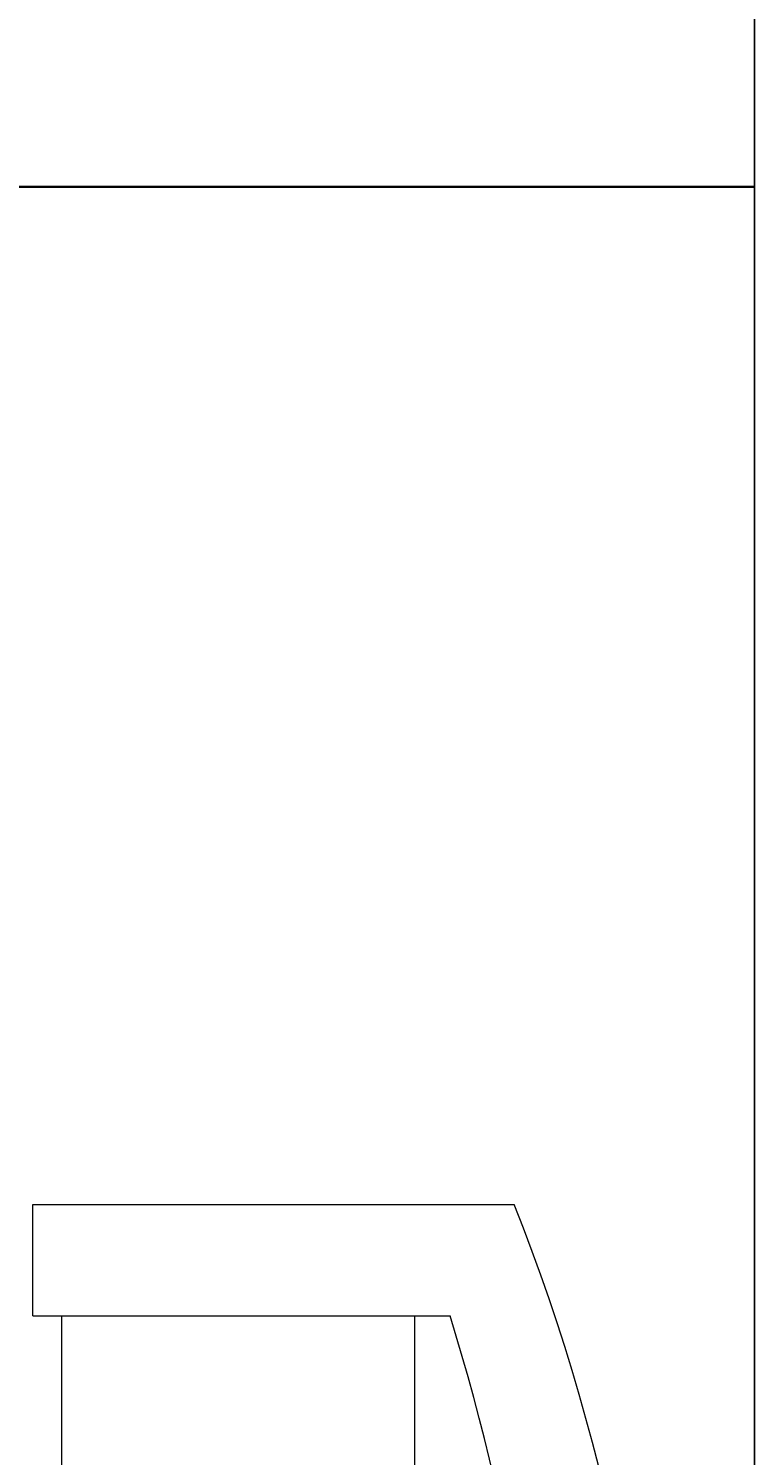
# Model space of a CAD drawing. Units: feet. Extents: x 1654 to 2985, y 1348 to 2230.
# Tile 51 of 53: x 2759 to 2785, y 1842 to 1892. Entities that reach past the tile are written whole.
import ezdxf

# ---------------------------------------------------------------- set-up
doc = ezdxf.new("R2010")
doc.units = ezdxf.units.FT
for name, color, linetype, lineweight in [('A-ANNO-DIMS', 2, 'Continuous', 18), ('A-FURN', 8, 'Continuous', 13), ('A-WALL', 7, 'Continuous', 35)]:
    doc.layers.add(name, color=color, linetype=linetype, lineweight=lineweight)
doc.styles.get("Standard").update_dxf_attribs({"font": 'arial.ttf'})
doc.dimstyles.get("Standard").update_dxf_attribs({"dimtxt": 0.18, "dimasz": 0.18, "dimexe": 0.18, "dimexo": 0.0625, "dimgap": 0.09, "dimtad": 0, "dimtih": 1, "dimtoh": 1, "dimdec": 4, "dimzin": 0, "dimdsep": 46, "dimtxsty": 'Standard', "dimcen": 0.09, "dimadec": 0, "dimazin": 0, "dimtfac": 1, "dimtdec": 4, "dimtofl": 0, "dimtmove": 0, "dimatfit": 3, "dimfxl": 1, "dimtolj": 1, "dimtzin": 0, "dimarcsym": 0})

# ---------------------------------------------------------------- blocks, each defined once
blk = doc.blocks.new('Sofa - Roundback 7 ft.')
for p, q in [((-36.000027, -34), (-36.000027, -11.4696)), ((-35.999844, -13.3819), (35.9998, -13.3819)), ((-36.000027, -32.4421), (35.99998, -32.4421))]:
    blk.add_line(p, q)
blk.add_lwpolyline([(-36.000027, -34), (-42.000027, -34), (-42.000027, -8)])
for centre, radius, start, end in [((0, -114.25), 114.25, 68.43141, 111.5686), ((-0.00001, -127.1968), 121.1968, 72.72033, 107.2797)]:
    blk.add_arc(centre, radius, start, end)
blk = doc.blocks.new('*D82')
at = {"layer": 'A-ANNO-DIMS', "color": 0, "lineweight": -2, "transparency": 16777216}
for p, q in [((2652.706, 2039.192), (2652.706, 1490.625)), ((2784.706, 2039.192), (2784.706, 1490.625)), ((2652.886, 1490.805), (2718.426, 1490.805)), ((2784.526, 1490.805), (2718.985, 1490.805))]:
    blk.add_line(p, q, dxfattribs=at)
at = {"layer": 'A-ANNO-DIMS', "color": 0, "transparency": 16777216}
for points in [[(2652.886, 1490.835), (2652.886, 1490.775), (2652.706, 1490.805)], [(2784.526, 1490.835), (2784.526, 1490.775), (2784.706, 1490.805)]]:
    blk.add_solid(points, dxfattribs=at)
at = {"layer": 'Defpoints', "color": 0, "transparency": 16777216}
for p in [(2652.706, 2039.255), (2784.706, 2039.255), (2784.706, 1490.805)]:
    blk.add_point(p, dxfattribs=at)
at = {"layer": 'A-ANNO-DIMS', "color": 0, "transparency": 16777216, "insert": (2718.706, 1490.805), "char_height": 0.18, "attachment_point": 5}
blk.add_mtext('\\A1;132', dxfattribs=at)
blk = doc.blocks.new('*D86')
at = {"layer": 'A-ANNO-DIMS', "color": 0, "lineweight": -2, "transparency": 16777216}
for p, q in [((2748.706, 1616.317), (2748.706, 2149.885)), ((2784.706, 1607.317), (2784.706, 2149.885)), ((2748.886, 2149.705), (2766.487, 2149.705)), ((2784.526, 2149.705), (2766.925, 2149.705))]:
    blk.add_line(p, q, dxfattribs=at)
at = {"layer": 'A-ANNO-DIMS', "color": 0, "transparency": 16777216}
for points in [[(2748.886, 2149.735), (2748.886, 2149.675), (2748.706, 2149.705)], [(2784.526, 2149.735), (2784.526, 2149.675), (2784.706, 2149.705)]]:
    blk.add_solid(points, dxfattribs=at)
at = {"layer": 'Defpoints', "color": 0, "transparency": 16777216}
for p in [(2784.706, 2149.705), (2748.706, 1616.255), (2784.706, 1607.255)]:
    blk.add_point(p, dxfattribs=at)
at = {"layer": 'A-ANNO-DIMS', "color": 0, "transparency": 16777216, "insert": (2766.706, 2149.705), "char_height": 0.18, "attachment_point": 5}
blk.add_mtext('\\A1;36', dxfattribs=at)

msp = doc.modelspace()

# ---------------------------------------------------------------- linework, layer by layer
at = {"layer": 'A-WALL'}
msp.add_line((2784.7058, 1886.2549), (2652.7058, 1886.2549), dxfattribs=at)

# ---------------------------------------------------------------- block references
at = {"layer": 'A-FURN', "xscale": 0.6464854603293951, "yscale": 0.6464854603293951, "zscale": 0.6464854603293951, "rotation": 270}
msp.add_blockref('Sofa - Roundback 7 ft.', (2781.495, 1823.581), dxfattribs=at)

# ---------------------------------------------------------------- dimensions: what is measured, and where the dimension line sits
at = {"layer": 'A-ANNO-DIMS'}
for base, p1, p2, picture, middle in [((2784.7058, 2149.7049), (2748.7058, 1616.2549), (2784.7058, 1607.2549), '*D86', (2766.7058, 2149.7049)), ((2784.7058, 1490.8049), (2652.7058, 2039.2549), (2784.7058, 2039.2549), '*D82', (2718.7058, 1490.8049))]:
    dim = msp.add_linear_dim(base=base, p1=p1, p2=p2, dimstyle='Standard', override={"dimdec": 0, "dimlfac": 1, "dimrnd": 0, "dimzin": 0, "dimdsep": 46, "dimlunit": 2}, dxfattribs=at)
    dim.commit()
    dim.dimension.update_dxf_attribs({"geometry": picture, "text_midpoint": middle})

doc.saveas('drawing.dxf')
